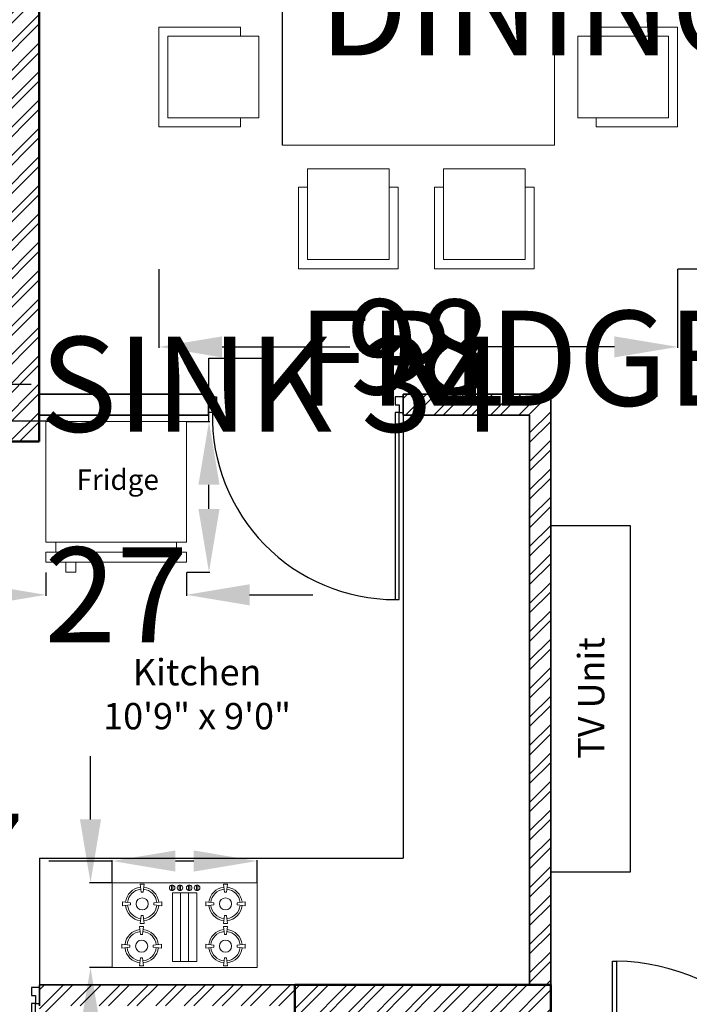
# Model space of a CAD drawing. Units: inches. Extents: x -90 to 536, y -553 to 299.
# Tile 12 of 27: x 79 to 206, y -339 to -153. Entities that reach past the tile are written whole.
import ezdxf

# ---------------------------------------------------------------- set-up
doc = ezdxf.new("R2010")
doc.units = ezdxf.units.IN
for name, color, linetype, lineweight in [('A-ANNO-DIMS', 2, 'Continuous', 18), ('A-ANNO-TEXT', 7, 'Continuous', 18), ('A-AREA-IDEN', 7, 'Continuous', 18), ('A-DOOR', 4, 'Continuous', 25), ('A-EQPM', 6, 'Continuous', 18), ('A-FLOR-CASE', 2, 'Continuous', 25), ('A-WALL-PATT', 252, 'Continuous', 13), ('Furniture', 2, 'Continuous', 18), ('Inner Wall', 5, 'Continuous', 35), ('Kitchen', 6, 'Continuous', 25), ('Outer Wall', 1, 'Continuous', 50)]:
    doc.layers.add(name, color=color, linetype=linetype, lineweight=lineweight)
doc.styles.get("Standard").update_dxf_attribs({"font": 'arial.ttf'})
doc.dimstyles.get("Standard").update_dxf_attribs({"dimtxt": 18, "dimasz": 12, "dimexe": 0.18, "dimexo": 0.0625, "dimgap": 0.09, "dimtad": 0, "dimtih": 1, "dimtoh": 1, "dimdec": 0, "dimzin": 0, "dimdsep": 46, "dimlunit": 3, "dimtxsty": 'Standard', "dimcen": 0.09, "dimadec": 0, "dimazin": 0, "dimtfac": 1, "dimtdec": 0, "dimtofl": 0, "dimtmove": 0, "dimatfit": 3, "dimfxl": 1, "dimtolj": 1, "dimtzin": 0, "dimarcsym": 0})

# ---------------------------------------------------------------- blocks, each defined once
blk = doc.blocks.new('A$C010165D4')
for p, q in [((0.7697, 2.4221), (0.7697, 2.8721)), ((0.7697, 2.8721), (1.3197, 2.8721)), ((0.8197, 2.8221), (0.8197, 2.3221)), ((1.2697, 2.8221), (0.8197, 2.8221)), ((1.2697, 2.3221), (1.2697, 2.8221)), ((1.3197, 2.8721), (1.3197, 2.4221)), ((1.5197, 2.4221), (1.5197, 2.8721)), ((1.5197, 2.8721), (2.0697, 2.8721)), ((1.5697, 2.8221), (1.5697, 2.3221)), ((2.0197, 2.8221), (1.5697, 2.8221)), ((2.0197, 2.3221), (2.0197, 2.8221)), ((2.0697, 2.8721), (2.0697, 2.4221)), ((0.8197, 2.4221), (0.7697, 2.4221)), ((1.3197, 2.4221), (1.2697, 2.4221)), ((1.5697, 2.4221), (1.5197, 2.4221)), ((2.0697, 2.4221), (2.0197, 2.4221)), ((1.2697, 2.3221), (0.8197, 2.3221)), ((2.0197, 2.3221), (1.5697, 2.3221)), ((0.6788, 2.1805), (0.6788, 0.6805)), ((0.6811, 0.6805), (0.6811, 2.1805)), ((0.6811, 2.1805), (2.1811, 2.1805)), ((2.1811, 2.1805), (2.1811, 0.6805)), ((0, 1.531), (0, 2.081)), ((0, 2.081), (0.45, 2.081)), ((0.45, 2.081), (0.45, 2.031)), ((2.8599, 2.081), (2.4099, 2.081)), ((2.4099, 2.081), (2.4099, 2.031)), ((2.8599, 1.531), (2.8599, 2.081)), ((0.05, 2.031), (0.05, 1.581)), ((0.55, 2.031), (0.05, 2.031)), ((0.55, 2.031), (0.55, 1.581)), ((2.3099, 2.031), (2.8099, 2.031)), ((2.3099, 2.031), (2.3099, 1.581)), ((2.8099, 2.031), (2.8099, 1.581)), ((0.05, 1.581), (0.55, 1.581)), ((0.45, 1.581), (0.45, 1.531)), ((2.8099, 1.581), (2.3099, 1.581)), ((2.4099, 1.581), (2.4099, 1.531)), ((0.45, 1.531), (0, 1.531)), ((2.4099, 1.531), (2.8599, 1.531)), ((0, 0.781), (0, 1.331)), ((0, 1.331), (0.45, 1.331)), ((0.45, 1.331), (0.45, 1.281)), ((2.4099, 1.331), (2.4099, 1.281)), ((2.8599, 1.331), (2.4099, 1.331)), ((2.8599, 0.781), (2.8599, 1.331)), ((0.05, 1.281), (0.05, 0.831)), ((0.55, 1.281), (0.05, 1.281)), ((0.55, 1.281), (0.55, 0.831)), ((2.3099, 1.281), (2.8099, 1.281)), ((2.3099, 1.281), (2.3099, 0.831)), ((2.8099, 1.281), (2.8099, 0.831)), ((0.05, 0.831), (0.55, 0.831)), ((0.45, 0.831), (0.45, 0.781)), ((2.8099, 0.831), (2.3099, 0.831)), ((2.4099, 0.831), (2.4099, 0.781)), ((0.45, 0.781), (0, 0.781)), ((2.4099, 0.781), (2.8599, 0.781)), ((2.1811, 0.6805), (0.6811, 0.6805)), ((0.8197, 0.05), (0.8197, 0.55)), ((1.2697, 0.55), (0.8197, 0.55)), ((1.2697, 0.55), (1.2697, 0.05)), ((1.5697, 0.05), (1.5697, 0.55)), ((2.0197, 0.55), (1.5697, 0.55)), ((2.0197, 0.55), (2.0197, 0.05)), ((0.7697, 0.45), (0.7697, 0)), ((0.8197, 0.45), (0.7697, 0.45)), ((1.3197, 0.45), (1.2697, 0.45)), ((1.3197, 0), (1.3197, 0.45)), ((1.5197, 0.45), (1.5197, 0)), ((1.5697, 0.45), (1.5197, 0.45)), ((2.0697, 0.45), (2.0197, 0.45)), ((2.0697, 0), (2.0697, 0.45)), ((1.2697, 0.05), (0.8197, 0.05)), ((2.0197, 0.05), (1.5697, 0.05)), ((0.7697, 0), (1.3197, 0)), ((1.5197, 0), (2.0697, 0))]:
    blk.add_line(p, q)
blk = doc.blocks.new('A$C57CF26DA')
for p, q in [((0, 0), (0, 420)), ((720, 420), (0, 420)), ((166.9, 413), (146.9, 413)), ((146.9, 413), (151.9, 373)), ((161.9, 373), (166.9, 413)), ((583.6, 413), (563.6, 413)), ((563.6, 413), (568.6, 373)), ((578.6, 373), (583.6, 413)), ((720, 0), (720, 420)), ((151.9, 373), (161.9, 373)), ((300, 390.9), (300, 49.1)), ((300, 390.9), (420, 390.9)), ((340, 390.9), (340, 49.1)), ((380, 390.9), (380, 49.1)), ((420, 390.9), (420, 49.1)), ((568.6, 373), (578.6, 373)), ((98.9, 320), (58.9, 325)), ((58.9, 325), (58.9, 305)), ((58.9, 305), (98.9, 310)), ((98.9, 310), (98.9, 320)), ((254.8, 325), (214.8, 320)), ((214.8, 320), (214.8, 310)), ((214.8, 310), (254.8, 305)), ((254.8, 305), (254.8, 325)), ((515.6, 320), (475.6, 325)), ((475.6, 325), (475.6, 305)), ((475.6, 305), (515.6, 310)), ((515.6, 310), (515.6, 320)), ((671.6, 325), (631.6, 320)), ((631.6, 320), (631.6, 310)), ((631.6, 310), (671.6, 305)), ((671.6, 305), (671.6, 325)), ((151.9, 257), (146.9, 217)), ((161.9, 257), (151.9, 257)), ((166.9, 217), (161.9, 257)), ((568.6, 257), (563.6, 217)), ((578.6, 257), (568.6, 257)), ((583.6, 217), (578.6, 257)), ((146.9, 217), (166.9, 217)), ((166.9, 203), (146.9, 203)), ((146.9, 203), (151.9, 163)), ((161.9, 163), (166.9, 203)), ((581.1, 203), (561.1, 203)), ((561.1, 203), (566.1, 163)), ((563.6, 217), (583.6, 217)), ((576.1, 163), (581.1, 203)), ((151.9, 163), (161.9, 163)), ((566.1, 163), (576.1, 163)), ((98.9, 110), (58.9, 115)), ((58.9, 115), (58.9, 95)), ((58.9, 95), (98.9, 100)), ((98.9, 100), (98.9, 110)), ((254.8, 115), (214.8, 110)), ((214.8, 110), (214.8, 100)), ((214.8, 100), (254.8, 95)), ((254.8, 95), (254.8, 115)), ((513.1, 110), (473.1, 115)), ((473.1, 115), (473.1, 95)), ((473.1, 95), (513.1, 100)), ((513.1, 100), (513.1, 110)), ((669, 115), (629, 110)), ((629, 110), (629, 100)), ((629, 100), (669, 95)), ((669, 95), (669, 115)), ((420, 49.1), (300, 49.1)), ((151.9, 47), (146.9, 7)), ((146.9, 7), (166.9, 7)), ((161.9, 47), (151.9, 47)), ((166.9, 7), (161.9, 47)), ((301.5, 38.7), (294.7, 38.7)), ((294.7, 38.7), (294.7, 11.3)), ((294.7, 11.3), (301.5, 11.3)), ((301.5, 11.3), (301.5, 38.7)), ((340.5, 38.7), (333.7, 38.7)), ((333.7, 38.7), (333.7, 11.3)), ((333.7, 11.3), (340.5, 11.3)), ((340.5, 11.3), (340.5, 38.7)), ((379.7, 11.3), (379.7, 38.7)), ((379.7, 38.7), (386.5, 38.7)), ((386.5, 11.3), (379.7, 11.3)), ((386.5, 38.7), (386.5, 11.3)), ((418.7, 11.3), (418.7, 38.7)), ((418.7, 38.7), (425.5, 38.7)), ((425.5, 11.3), (418.7, 11.3)), ((425.5, 38.7), (425.5, 11.3)), ((566.1, 47), (561.1, 7)), ((561.1, 7), (581.1, 7)), ((576.1, 47), (566.1, 47)), ((581.1, 7), (576.1, 47)), ((720, 0), (0, 0))]:
    blk.add_line(p, q)
for centre in [(156.9, 315), (573.6, 315), (156.9, 105), (571.1, 105)]:
    blk.add_circle(centre, 30)
for centre, radius, start, end in [((156.9, 315), 83, 95.5849, 174.4151), ((156.9, 315), 83, 5.5849, 84.4151), ((573.6, 315), 83, 95.5849, 174.4151), ((573.6, 315), 83, 5.5849, 84.4151), ((156.9, 315), 73, 95.3738, 174.6262), ((156.9, 315), 73, 5.3738, 84.6262), ((573.6, 315), 73, 95.3738, 174.6262), ((573.6, 315), 73, 5.3738, 84.6262), ((156.9, 315), 83, 185.5849, 264.4151), ((156.9, 315), 73, 185.3738, 264.6262), ((156.9, 315), 73, 275.3738, 354.6262), ((156.9, 315), 83, 275.5849, 354.4151), ((573.6, 315), 83, 185.5849, 264.4151), ((573.6, 315), 73, 185.3738, 264.6262), ((573.6, 315), 73, 275.3738, 354.6262), ((573.6, 315), 83, 275.5849, 354.4151), ((156.9, 105), 83, 95.5849, 174.4151), ((156.9, 105), 73, 95.3738, 174.6262), ((156.9, 105), 73, 5.3738, 84.6262), ((156.9, 105), 83, 5.5849, 84.4151), ((571.1, 105), 83, 95.5849, 174.4151), ((571.1, 105), 73, 95.3738, 174.6262), ((571.1, 105), 73, 5.3738, 84.6262), ((571.1, 105), 83, 5.5849, 84.4151), ((156.9, 105), 73, 185.3738, 264.6262), ((156.9, 105), 73, 275.3738, 354.6262), ((571.1, 105), 73, 185.3738, 264.6262), ((571.1, 105), 73, 275.3738, 354.6262), ((156.9, 105), 83, 185.5849, 264.4151), ((156.9, 105), 83, 275.5849, 354.4151), ((571.1, 105), 83, 185.5849, 264.4151), ((571.1, 105), 83, 275.5849, 354.4151), ((298.1, 25), 13.7, 104.4775, 255.5225), ((298.1, 25), 13.7, 284.4775, 75.5225), ((337.1, 25), 13.7, 104.4775, 255.5225), ((337.1, 25), 13.7, 284.4775, 75.5225), ((383.1, 25), 13.7, 104.4775, 255.5225), ((383.1, 25), 13.7, 284.4775, 75.5225), ((422.1, 25), 13.7, 104.4775, 255.5225), ((422.1, 25), 13.7, 284.4775, 75.5225)]:
    blk.add_arc(centre, radius, start, end)
blk = doc.blocks.new('REFRI-00')
for points in [[(-0.35, 0.35), (-0.35, -0.25), (0.35, -0.25), (0.35, 0.35), (-0.35, 0.35)], [(-0.3, -0.3), (-0.3, -0.25)], [(0.3, -0.3), (0.3, -0.25)], [(-0.35, -0.3), (-0.35, -0.35), (0.35, -0.35), (0.35, -0.3), (-0.35, -0.3)], [(-0.25, -0.35), (-0.25, -0.4), (-0.2, -0.4), (-0.2, -0.35)]]:
    blk.add_lwpolyline(points)
blk = doc.blocks.new('DOOR-36-A')
for points in [[(35.25, 37.5), (35.25, 3), (34.5, 3), (34.5, 37.5)], [(0, 0), (1.5, 0), (1.5, 1.5), (0.75, 1.5), (0.75, 3), (0, 3)], [(36, 0), (34.5, 0), (34.5, 1.5), (35.25, 1.5), (35.25, 3), (36, 3)]]:
    blk.add_lwpolyline(points, close=True)
blk.add_arc((37.64, 1.5), 36.14, 94.9791, 180)
blk = doc.blocks.new('DOOR-42')
for points in [[(0.75, 3), (0.75, 43.5), (1.5, 43.5), (1.5, 3)], [(0, 0), (1.5, 0), (1.5, 1.5), (0.75, 1.5), (0.75, 3), (0, 3)], [(42, 0), (40.5, 0), (40.5, 1.5), (41.25, 1.5), (41.25, 3), (42, 3)]]:
    blk.add_lwpolyline(points, close=True)
blk.add_arc((0.74, 3), 40.51, 0, 88.9291)
blk = doc.blocks.new('TV-UNIT')
blk.add_lwpolyline([(15, 65.77), (15, 0), (0, 0), (0, 65.77)], close=True)
blk = doc.blocks.new('*D35')
at = {"layer": 'A-ANNO-DIMS', "color": 0, "lineweight": -2, "transparency": 16777216}
for p, q in [((233.19, -331.05), (239.84, -331.05)), ((239.66, -343.05), (239.66, -343.4)), ((239.66, -362.55), (239.66, -362.21)), ((233.19, -374.55), (239.84, -374.55))]:
    blk.add_line(p, q, dxfattribs=at)
at = {"layer": 'A-ANNO-DIMS', "color": 0, "transparency": 16777216}
for points in [[(237.66, -343.05), (241.66, -343.05), (239.66, -331.05)], [(237.66, -362.55), (241.66, -362.55), (239.66, -374.55)]]:
    blk.add_solid(points, dxfattribs=at)
at = {"layer": 'Defpoints', "color": 0, "transparency": 16777216}
for p in [(233.13, -331.05), (239.66, -331.05), (233.13, -374.55)]:
    blk.add_point(p, dxfattribs=at)
at = {"layer": 'A-ANNO-DIMS', "color": 0, "transparency": 16777216, "insert": (239.66, -352.8), "char_height": 18, "attachment_point": 5}
blk.add_mtext('\\A1;ENTRY DOOR 44 TYP.', dxfattribs=at)
blk = doc.blocks.new('*D41')
at = {"layer": 'A-ANNO-DIMS', "color": 0, "lineweight": -2, "transparency": 16777216}
for p, q in [((204.27, -100.92), (219.21, -100.92)), ((219.03, -112.92), (219.03, -140.95)), ((219.03, -187.77), (219.03, -159.74)), ((204.27, -199.77), (219.21, -199.77))]:
    blk.add_line(p, q, dxfattribs=at)
at = {"layer": 'A-ANNO-DIMS', "color": 0, "transparency": 16777216}
for points in [[(217.03, -112.92), (221.03, -112.92), (219.03, -100.92)], [(217.03, -187.77), (221.03, -187.77), (219.03, -199.77)]]:
    blk.add_solid(points, dxfattribs=at)
at = {"layer": 'Defpoints', "color": 0, "transparency": 16777216}
for p in [(204.21, -100.92), (219.03, -100.92), (204.21, -199.77)]:
    blk.add_point(p, dxfattribs=at)
at = {"layer": 'A-ANNO-DIMS', "color": 0, "transparency": 16777216, "insert": (219.03, -150.34), "char_height": 18, "attachment_point": 5}
blk.add_mtext('\\A1;DINING SET 99', dxfattribs=at)
blk = doc.blocks.new('*D42')
at = {"layer": 'A-ANNO-DIMS', "color": 0, "lineweight": -2, "transparency": 16777216}
for p, q in [((105.78, -199.83), (105.78, -214.77)), ((204.21, -199.83), (204.21, -214.77)), ((117.78, -214.59), (142, -214.59)), ((192.21, -214.59), (168, -214.59))]:
    blk.add_line(p, q, dxfattribs=at)
at = {"layer": 'A-ANNO-DIMS', "color": 0, "transparency": 16777216}
for points in [[(117.78, -212.59), (117.78, -216.59), (105.78, -214.59)], [(192.21, -212.59), (192.21, -216.59), (204.21, -214.59)]]:
    blk.add_solid(points, dxfattribs=at)
at = {"layer": 'Defpoints', "color": 0, "transparency": 16777216}
for p in [(105.78, -199.77), (204.21, -199.77), (204.21, -214.59)]:
    blk.add_point(p, dxfattribs=at)
at = {"layer": 'A-ANNO-DIMS', "color": 0, "transparency": 16777216, "insert": (155, -214.59), "char_height": 18, "attachment_point": 5}
blk.add_mtext('\\A1;98', dxfattribs=at)
blk = doc.blocks.new('*D45')
at = {"layer": 'A-ANNO-DIMS', "color": 0, "lineweight": -2, "transparency": 16777216}
for p, q in [((96.92, -312.07), (84.92, -312.07)), ((96.92, -316.13), (96.92, -311.89)), ((112.4, -312.07), (108.92, -312.07)), ((124.4, -316.13), (124.4, -311.89))]:
    blk.add_line(p, q, dxfattribs=at)
at = {"layer": 'A-ANNO-DIMS', "color": 0, "transparency": 16777216}
for points in [[(108.92, -310.07), (108.92, -314.07), (96.92, -312.07)], [(112.4, -310.07), (112.4, -314.07), (124.4, -312.07)]]:
    blk.add_solid(points, dxfattribs=at)
at = {"layer": 'Defpoints', "color": 0, "transparency": 16777216}
for p in [(96.92, -312.07), (96.92, -316.19), (124.4, -316.19)]:
    blk.add_point(p, dxfattribs=at)
at = {"layer": 'A-ANNO-DIMS', "color": 0, "transparency": 16777216, "insert": (5.68, -312.07), "char_height": 18, "attachment_point": 5}
blk.add_mtext('\\A1;COOKTOP 27', dxfattribs=at)
blk = doc.blocks.new('*D46')
at = {"layer": 'A-ANNO-DIMS', "color": 0, "lineweight": -2, "transparency": 16777216}
for p, q in [((92.8, -304.19), (92.8, -292.19)), ((96.86, -316.19), (92.62, -316.19)), ((96.86, -332.23), (92.62, -332.23)), ((92.8, -344.23), (92.8, -356.23)), ((92.8, -356.23), (80.8, -356.23))]:
    blk.add_line(p, q, dxfattribs=at)
at = {"layer": 'A-ANNO-DIMS', "color": 0, "transparency": 16777216}
for points in [[(90.8, -304.19), (94.8, -304.19), (92.8, -316.19)], [(90.8, -344.23), (94.8, -344.23), (92.8, -332.23)]]:
    blk.add_solid(points, dxfattribs=at)
at = {"layer": 'Defpoints', "color": 0, "transparency": 16777216}
for p in [(96.92, -316.19), (92.8, -332.23), (96.92, -332.23)]:
    blk.add_point(p, dxfattribs=at)
at = {"layer": 'A-ANNO-DIMS', "color": 0, "transparency": 16777216, "insert": (68.67, -356.23), "char_height": 18, "attachment_point": 5}
blk.add_mtext('\\A1;16', dxfattribs=at)
blk = doc.blocks.new('*D47')
at = {"layer": 'A-ANNO-DIMS', "color": 0, "lineweight": -2, "transparency": 16777216}
for p, q in [((69.57, -233.68), (69.57, -221.68)), ((69.57, -221.68), (81.57, -221.68)), ((64.53, -233.68), (69.75, -233.68)), ((69.57, -255.69), (69.57, -245.68)), ((64.53, -267.69), (69.75, -267.69))]:
    blk.add_line(p, q, dxfattribs=at)
at = {"layer": 'A-ANNO-DIMS', "color": 0, "transparency": 16777216}
for points in [[(67.57, -245.68), (71.57, -245.68), (69.57, -233.68)], [(67.57, -255.69), (71.57, -255.69), (69.57, -267.69)]]:
    blk.add_solid(points, dxfattribs=at)
at = {"layer": 'Defpoints', "color": 0, "transparency": 16777216}
for p in [(64.47, -233.68), (69.57, -233.68), (64.47, -267.69)]:
    blk.add_point(p, dxfattribs=at)
at = {"layer": 'A-ANNO-DIMS', "color": 0, "transparency": 16777216, "insert": (127.31, -221.68), "char_height": 18, "attachment_point": 5}
blk.add_mtext('\\A1;SINK 34', dxfattribs=at)
blk = doc.blocks.new('*D48')
at = {"layer": 'A-ANNO-DIMS', "color": 0, "lineweight": -2, "transparency": 16777216}
for p, q in [((36.62, -228.58), (24.62, -228.58)), ((48.62, -233.62), (48.62, -228.4)), ((64.47, -233.62), (64.47, -228.4)), ((76.47, -228.58), (88.47, -228.58))]:
    blk.add_line(p, q, dxfattribs=at)
at = {"layer": 'A-ANNO-DIMS', "color": 0, "transparency": 16777216}
for points in [[(36.62, -226.58), (36.62, -230.58), (48.62, -228.58)], [(76.47, -226.58), (76.47, -230.58), (64.47, -228.58)]]:
    blk.add_solid(points, dxfattribs=at)
at = {"layer": 'Defpoints', "color": 0, "transparency": 16777216}
for p in [(48.62, -228.58), (48.62, -233.68), (64.47, -233.68)]:
    blk.add_point(p, dxfattribs=at)
at = {"layer": 'A-ANNO-DIMS', "color": 0, "transparency": 16777216, "insert": (12.5, -228.58), "char_height": 18, "attachment_point": 5}
blk.add_mtext('\\A1;16', dxfattribs=at)
blk = doc.blocks.new('*D49')
at = {"layer": 'A-ANNO-DIMS', "color": 0, "lineweight": -2, "transparency": 16777216}
for p, q in [((115.28, -228.74), (115.28, -216.74)), ((115.28, -216.74), (127.28, -216.74)), ((111.06, -228.74), (115.46, -228.74)), ((115.28, -245.31), (115.28, -240.74)), ((111.06, -257.31), (115.46, -257.31))]:
    blk.add_line(p, q, dxfattribs=at)
at = {"layer": 'A-ANNO-DIMS', "color": 0, "transparency": 16777216}
for points in [[(113.28, -240.74), (117.28, -240.74), (115.28, -228.74)], [(113.28, -245.31), (117.28, -245.31), (115.28, -257.31)]]:
    blk.add_solid(points, dxfattribs=at)
at = {"layer": 'Defpoints', "color": 0, "transparency": 16777216}
for p in [(111, -228.74), (115.28, -228.74), (111, -257.31)]:
    blk.add_point(p, dxfattribs=at)
at = {"layer": 'A-ANNO-DIMS', "color": 0, "transparency": 16777216, "insert": (190.77, -216.74), "char_height": 18, "attachment_point": 5}
blk.add_mtext('\\A1;FRIDGE 29', dxfattribs=at)
blk = doc.blocks.new('*D50')
at = {"layer": 'A-ANNO-DIMS', "color": 0, "lineweight": -2, "transparency": 16777216}
for p, q in [((84.33, -257.38), (84.33, -261.78)), ((111, -257.38), (111, -261.78)), ((72.33, -261.6), (60.33, -261.6)), ((123, -261.6), (135, -261.6))]:
    blk.add_line(p, q, dxfattribs=at)
at = {"layer": 'A-ANNO-DIMS', "color": 0, "transparency": 16777216}
for points in [[(72.33, -259.6), (72.33, -263.6), (84.33, -261.6)], [(123, -259.6), (123, -263.6), (111, -261.6)]]:
    blk.add_solid(points, dxfattribs=at)
at = {"layer": 'Defpoints', "color": 0, "transparency": 16777216}
for p in [(84.33, -257.31), (111, -257.31), (111, -261.6)]:
    blk.add_point(p, dxfattribs=at)
at = {"layer": 'A-ANNO-DIMS', "color": 0, "transparency": 16777216, "insert": (97.67, -261.6), "char_height": 18, "attachment_point": 5}
blk.add_mtext('\\A1;27', dxfattribs=at)
blk = doc.blocks.new('*D54')
at = {"layer": 'A-ANNO-DIMS', "color": 0, "lineweight": -2, "transparency": 16777216}
for p, q in [((113.07, 249.45), (-2.85, 249.45)), ((-2.67, 237.45), (-2.67, -117.77)), ((-2.67, -491.55), (-2.67, -136.34)), ((38.07, -503.55), (-2.85, -503.55))]:
    blk.add_line(p, q, dxfattribs=at)
at = {"layer": 'A-ANNO-DIMS', "color": 0, "transparency": 16777216}
for points in [[(-4.67, 237.45), (-0.67, 237.45), (-2.67, 249.45)], [(-4.67, -491.55), (-0.67, -491.55), (-2.67, -503.55)]]:
    blk.add_solid(points, dxfattribs=at)
at = {"layer": 'Defpoints', "color": 0, "transparency": 16777216}
for p in [(-2.67, 249.45), (113.13, 249.45), (38.13, -503.55)]:
    blk.add_point(p, dxfattribs=at)
at = {"layer": 'A-ANNO-DIMS', "color": 0, "transparency": 16777216, "insert": (-2.67, -127.05), "char_height": 18, "attachment_point": 5}
blk.add_mtext('\\A1;753', dxfattribs=at)

msp = doc.modelspace()

# ---------------------------------------------------------------- hatches: boundary and pattern name
at = {"layer": 'A-WALL-PATT'}
h = msp.add_hatch(dxfattribs=at)
h.set_pattern_fill('ANSI32', color=256, scale=0.4)
h.set_pattern_definition([(45, (-88.8105, -603.6155), (-2.694077, 2.694077), []), (45, (-87.0145, -603.6155), (-2.694077, 2.694077), [])])
h.paths.add_polyline_path([(285.1317, 246.4462), (131.1317, 246.4462), (131.1317, 237.4462), (285.1317, 237.4462)])
h.paths.add_polyline_path([(122.1317, 237.4462), (113.1317, 237.4462), (113.1317, 152.4462), (122.1317, 152.4462), (122.1317, 166.4704)])
h.paths.add_polyline_path([(303.1317, 237.4462), (294.1317, 237.4462), (294.1317, 152.4462), (303.1317, 152.4462)])
h.paths.add_polyline_path([(47.1317, 91.9277), (38.1317, 91.9277), (38.1317, -6.5538), (77.1317, -6.5538), (77.1317, 2.4462), (70.5655, 2.4462), (47.1317, 2.4462)])
h.paths.add_polyline_path([(83.052, -61.5538), (47.1317, -61.5538), (47.1317, -24.5538), (38.1317, -24.5538), (38.1317, -70.5538), (74.052, -70.5538), (74.052, -223.5538), (38.1317, -223.5538), (38.1317, -503.5538), (92.1317, -503.5538), (92.1317, -437.5538), (191.1317, -437.5538), (191.1317, -428.5538), (83.1317, -428.5538), (83.1317, -494.5538), (47.1317, -494.5538), (47.1317, -232.5538), (83.052, -232.5538), (83.052, -70.5538)])
h.paths.add_polyline_path([(407.1317, -63.5538), (381.1317, -63.5538), (381.1317, 91.9277), (372.1317, 91.9277), (372.1317, 32.8805), (372.1317, -63.5538), (306.5745, -63.5538), (237.1317, -63.5538), (237.1317, -38.5538), (233.1317, -38.5538), (233.1317, -71.5538), (398.1317, -71.5538), (398.1317, -152.5538), (233.1317, -152.5538), (233.1317, -161.5538), (398.1317, -161.5538), (398.1317, -368.5538), (233.1317, -368.5538), (233.1317, -377.5538), (407.1317, -377.5538), (407.1317, -161.5538)])
h.paths.add_polyline_path([(261.1317, -422.5538), (252.1317, -422.5538), (252.1317, -428.5538), (233.1317, -428.5538), (233.1317, -437.5538), (261.1317, -437.5538)])
h.paths.add_polyline_path([(191.1317, -368.5538), (180.1317, -368.5538), (180.1317, -335.5538), (131.5919, -335.5538), (131.5919, -344.5538), (171.1317, -344.5538), (171.1317, -392.5538), (180.1317, -392.5538), (180.1317, -377.5538), (191.1317, -377.5538)], flags=17)
h.paths.add_polyline_path([(180.1317, -223.5538), (152.1317, -223.5538), (152.1317, -227.5538), (176.1317, -227.5538), (176.1317, -335.5538), (180.1317, -335.5538)], flags=17)
h.paths.add_polyline_path([(131.5919, -335.5538), (83.1317, -335.5538), (83.1317, -339.5538), (83.1317, -392.5538), (87.1317, -392.5538), (87.1317, -339.5538), (131.5919, -339.5538)], flags=17)
h.paths.add_polyline_path([(197.1317, 2.4462), (77.1317, 2.4462), (77.1317, -1.5538), (113.1317, -1.5538), (113.1317, -71.5538), (181.1317, -71.5538), (181.1317, -67.5538), (117.1317, -67.5538), (117.1317, -1.5538), (177.1317, -1.5538), (177.1317, -37.5538), (181.1317, -37.5538), (181.1317, -1.5538), (197.1317, -1.5538)])
h.paths.add_polyline_path([(173.1317, 138.4462), (122.1317, 138.4462), (122.1317, 134.4462), (173.1317, 134.4462)])
h.paths.add_polyline_path([(213.1317, 237.4462), (209.1317, 237.4462), (209.1317, 134.4462), (233.1317, 134.4462), (233.1317, 68.8889), (233.1317, -2.5538), (237.1317, -2.5538), (237.1317, 134.4462), (258.1317, 134.4462), (258.1317, 138.4462), (213.1317, 138.4462)])

# ---------------------------------------------------------------- linework, layer by layer
at = {"layer": 'A-DOOR'}
for points in [[(115.1887, -224.0538), (116.6887, -224.0538), (116.6887, -225.5538), (115.9387, -225.5538), (115.9387, -227.0538), (115.1887, -227.0538)], [(152.1317, -224.0538), (150.6317, -224.0538), (150.6317, -225.5538), (151.3817, -225.5538), (151.3817, -227.0538), (152.1317, -227.0538)], [(151.3817, -262.4969), (151.3817, -227.0538), (150.6317, -227.0538), (150.6317, -262.4969)]]:
    msp.add_lwpolyline(points, close=True, dxfattribs=at)
msp.add_arc((150.6317, -227.7958), 34.701, 178.774664, 270, dxfattribs=at)
at = {"layer": 'Inner Wall'}
for p, q in [((83.052, -223.5538), (115.1887, -223.5538)), ((115.1887, -223.5538), (115.1887, -227.5538)), ((152.1317, -223.5538), (152.1317, -227.5538)), ((152.1317, -223.5538), (180.1317, -223.5538)), ((180.1317, -223.5538), (180.1317, -335.5538)), ((83.052, -227.5538), (115.1887, -227.5538)), ((152.1317, -227.5538), (176.1317, -227.5538)), ((176.1317, -227.5538), (176.1317, -335.5538)), ((83.1317, -335.5538), (180.1317, -335.5538)), ((83.1317, -339.5538), (83.1317, -335.5538))]:
    msp.add_line(p, q, dxfattribs=at)
at = {"layer": 'Kitchen'}
for p, q in [((152.1317, -227.5538), (152.1317, -311.5538)), ((176.1317, -227.5538), (152.1317, -227.5538)), ((176.1317, -335.5538), (176.1317, -227.5538)), ((83.1317, -311.5538), (152.1317, -311.5538)), ((83.1317, -311.5538), (83.1317, -335.5538)), ((83.1317, -335.5538), (176.1317, -335.5538))]:
    msp.add_line(p, q, dxfattribs=at)
at = {"layer": 'Outer Wall'}
for p, q in [((83.052, -70.5538), (83.052, -232.5538)), ((83.052, -232.5538), (47.1317, -232.5538)), ((180.1317, -335.5538), (131.5919, -335.5538)), ((131.5919, -335.5538), (131.5919, -344.5538)), ((180.1317, -368.5538), (180.1317, -335.5538))]:
    msp.add_line(p, q, dxfattribs=at)

# ---------------------------------------------------------------- block references
at = {"layer": 'A-DOOR'}
msp.add_blockref('DOOR-42', (191.1317, -374.5538), dxfattribs=at)
at = {"layer": 'A-DOOR', "extrusion": (0, 0, -1), "zscale": -1, "rotation": 180}
msp.add_blockref('DOOR-36-A', (-47.1317, -336.0538), dxfattribs=at)
at = {"layer": 'A-EQPM', "xscale": 38.0932829071003, "yscale": 38.0932829071003, "zscale": 38.0932829071003}
msp.add_blockref('REFRI-00', (97.6662, -242.0774), dxfattribs=at)
at = {"layer": 'A-EQPM', "xscale": 0.0381707681172169, "yscale": 0.0381707681172169, "zscale": 0.0381707681172169, "rotation": 180}
msp.add_blockref('A$C57CF26DA', (124.4017, -316.194), dxfattribs=at)
at = {"layer": 'A-FLOR-CASE', "rotation": 180}
msp.add_blockref('TV-UNIT', (195.2316, -248.4294), dxfattribs=at)
at = {"layer": 'Furniture', "xscale": 34.41518617011034, "yscale": 34.41518617011034, "zscale": 34.41518617011034}
msp.add_blockref('A$C010165D4', (105.7848, -199.766), dxfattribs=at)

# ---------------------------------------------------------------- texts
at = {"layer": 'A-ANNO-TEXT', "insert": (88.9914, -237.8216), "char_height": 3.877971, "attachment_point": 1}
msp.add_mtext_dynamic_manual_height_columns('\\pxqc;{\\fTimes New Roman|b0|i0|c0|p18;Fridge}', width=17.951771, gutter_width=4.8475, heights=[0], dxfattribs=at)
at = {"layer": 'A-ANNO-TEXT', "insert": (185.301, -263.5281), "char_height": 5, "attachment_point": 3, "rotation": 90}
msp.add_mtext_dynamic_manual_height_columns('\\pxqc;{\\fTimes New Roman|b0|i0|c0|p18;TV Unit}', width=35.23368, gutter_width=12.5, heights=[0], dxfattribs=at)
at = {"layer": 'A-AREA-IDEN', "insert": (137.7038, -273.7659), "char_height": 5, "attachment_point": 3}
msp.add_mtext_dynamic_manual_height_columns('\\pxqc;{\\fTimes New Roman|b0|i0|c0|p18;Kitchen\\P10\'9" x 9\'0"}', width=49.342153, gutter_width=12.5, heights=[0], dxfattribs=at)

# ---------------------------------------------------------------- dimensions: what is measured, and where the dimension line sits
at = {"layer": 'A-ANNO-DIMS'}
for base, p1, p2, angle, picture, middle in [((-2.6677, 249.4462), (38.1317, -503.5538), (113.1317, 249.4462), 90, '*D54', (-2.6677, -127.0538)), ((48.6244, -228.5837), (64.4668, -233.6849), (48.6244, -233.6849), 180, '*D48', (12.4955, -228.5837)), ((92.7963, -332.2258), (96.9187, -316.194), (96.9187, -332.2258), 270, '*D46', (68.6674, -356.2258))]:
    dim = msp.add_linear_dim(base=base, p1=p1, p2=p2, angle=angle, dimstyle='Standard', override={"dimdec": 0, "dimlfac": 1, "dimrnd": 0, "dimzin": 0, "dimdsep": 46, "dimlunit": 2}, dxfattribs=at)
    dim.commit()
    dim.dimension.update_dxf_attribs({"geometry": picture, "text_midpoint": middle})
for base, p1, p2, angle, text, picture, middle in [((219.0345, -100.9205), (204.2077, -199.766), (204.2077, -100.9205), 90, 'DINING SET <>', '*D41', (219.0345, -150.3432)), ((115.2843, -228.7447), (110.9988, -257.3147), (110.9988, -228.7447), 90, 'FRIDGE <>', '*D49', (190.7672, -216.7447)), ((69.5681, -233.6849), (64.4668, -267.6933), (64.4668, -233.6849), 90, 'SINK <>', '*D47', (127.3088, -221.6849)), ((96.9187, -312.0716), (124.4017, -316.194), (96.9187, -316.194), 180, 'COOKTOP <>', '*D45', (5.6766, -312.0716)), ((239.6567404714, -331.0537825705), (233.1317404714, -374.5537825705), (233.1317404714, -331.0537825705), 90, 'ENTRY DOOR <> TYP.', '*D35', (239.6567404714, -352.8037825705))]:
    dim = msp.add_linear_dim(base=base, p1=p1, p2=p2, angle=angle, text=text, dimstyle='Standard', override={"dimdec": 0, "dimlfac": 1, "dimrnd": 0, "dimzin": 0, "dimdsep": 46, "dimlunit": 2}, dxfattribs=at)
    dim.commit()
    dim.dimension.update_dxf_attribs({"geometry": picture, "text_midpoint": middle})
for base, p1, p2, picture, middle in [((204.2077, -214.5928), (105.7848, -199.766), (204.2077, -199.766), '*D42', (154.9962, -214.5928)), ((110.9988, -261.6002), (84.3335, -257.3147), (110.9988, -257.3147), '*D50', (97.6662, -261.6002))]:
    dim = msp.add_linear_dim(base=base, p1=p1, p2=p2, dimstyle='Standard', override={"dimdec": 0, "dimlfac": 1, "dimrnd": 0, "dimzin": 0, "dimdsep": 46, "dimlunit": 2}, dxfattribs=at)
    dim.commit()
    dim.dimension.update_dxf_attribs({"geometry": picture, "text_midpoint": middle})

doc.saveas('drawing.dxf')
